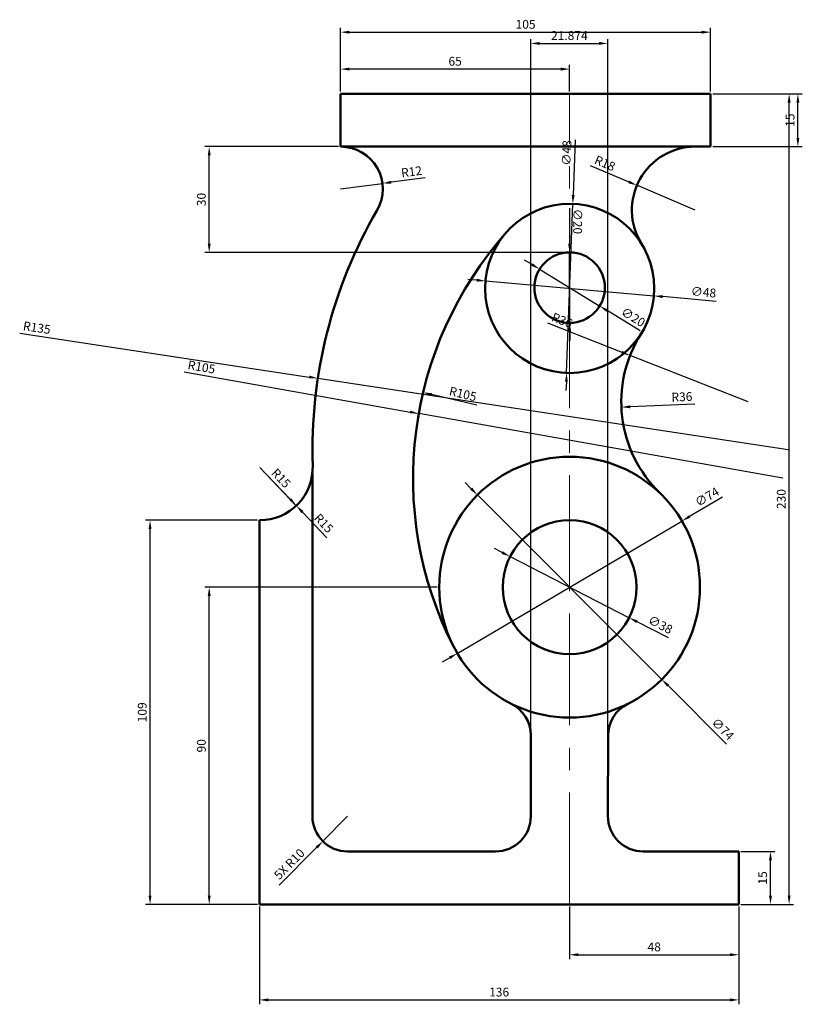
# Model space of a CAD drawing. Units: millimetres. Extents: x 3631 to 150643, y 1395 to 1701.
# Tile 1 of 1: x 3631.2 to 3853.3, y 1421.4 to 1700.8. Entities that reach past the tile are written whole.
import ezdxf

# ---------------------------------------------------------------- set-up
doc = ezdxf.new("R2010")
doc.units = ezdxf.units.MM
doc.linetypes.add('CENTER', pattern=[50.8, 31.75, -6.35, 6.35, -6.35])
for name, color, linetype, lineweight in [('M-CNTR', 4, 'CENTER', 18), ('M-CONS', 8, 'Continuous', 13), ('M-DIMS', 2, 'Continuous', 25), ('M-OUTL', 7, 'Continuous', 50)]:
    doc.layers.add(name, color=color, linetype=linetype, lineweight=lineweight)
doc.styles.get("Standard").update_dxf_attribs({"font": 'arial.ttf'})
doc.dimstyles.new('ISO-25', dxfattribs={"dimtxt": 2.5, "dimasz": 2.5, "dimexe": 1.25, "dimexo": 0.625, "dimtad": 1, "dimtxsty": 'Standard', "dimcen": 2.5, "dimadec": 0, "dimazin": 0, "dimtfac": 1, "dimtmove": 0, "dimatfit": 3, "dimfxl": 1, "dimarcsym": 0})

# ---------------------------------------------------------------- blocks, each defined once
blk = doc.blocks.new('*D1')
at = {"layer": 'Defpoints', "color": 0, "transparency": 16777216}
for p in [(3819.18, 1558.53), (3755.41, 1520.98)]:
    blk.add_point(p, dxfattribs=at)
at = {"layer": 'M-DIMS', "color": 0, "lineweight": -2, "transparency": 16777216}
for p, q in [((3830.7, 1565.31), (3821.33, 1559.79)), ((3755.41, 1520.98), (3819.18, 1558.53)), ((3753.26, 1519.71), (3751.1, 1518.44))]:
    blk.add_line(p, q, dxfattribs=at)
at = {"layer": 'M-DIMS', "color": 0, "transparency": 16777216}
for points in [[(3821.12, 1560.15), (3821.54, 1559.44), (3819.18, 1558.53)], [(3753.04, 1520.07), (3753.47, 1519.35), (3755.41, 1520.98)]]:
    blk.add_solid(points, dxfattribs=at)
at = {"layer": 'M-DIMS', "color": 0, "transparency": 16777216, "insert": (3826.45, 1565.1), "char_height": 2.5, "attachment_point": 5, "rotation": 30.49}
blk.add_mtext('∅74', dxfattribs=at)
blk = doc.blocks.new('*D2')
at = {"layer": 'Defpoints', "color": 0, "transparency": 16777216}
for p in [(3770.39, 1548.43), (3804.2, 1531.08)]:
    blk.add_point(p, dxfattribs=at)
at = {"layer": 'M-DIMS', "color": 0, "lineweight": -2, "transparency": 16777216}
for p, q in [((3768.16, 1549.57), (3765.94, 1550.71)), ((3770.39, 1548.43), (3804.2, 1531.08)), ((3815.37, 1525.35), (3806.42, 1529.94))]:
    blk.add_line(p, q, dxfattribs=at)
at = {"layer": 'M-DIMS', "color": 0, "transparency": 16777216}
for points in [[(3768.35, 1549.94), (3767.97, 1549.2), (3770.39, 1548.43)], [(3806.61, 1530.31), (3806.23, 1529.57), (3804.2, 1531.08)]]:
    blk.add_solid(points, dxfattribs=at)
at = {"layer": 'M-DIMS', "color": 0, "transparency": 16777216, "insert": (3812.91, 1528.83), "char_height": 2.5, "attachment_point": 5, "rotation": 332.8421}
blk.add_mtext('∅38', dxfattribs=at)
blk = doc.blocks.new('*D3')
at = {"layer": 'Defpoints', "color": 0, "transparency": 16777216}
for p in [(3778.77, 1629.98), (3795.82, 1619.53)]:
    blk.add_point(p, dxfattribs=at)
at = {"layer": 'M-DIMS', "color": 0, "lineweight": -2, "transparency": 16777216}
for p, q in [((3776.64, 1631.29), (3774.51, 1632.59)), ((3778.77, 1629.98), (3795.82, 1619.53)), ((3807.34, 1612.46), (3797.95, 1618.22))]:
    blk.add_line(p, q, dxfattribs=at)
at = {"layer": 'M-DIMS', "color": 0, "transparency": 16777216}
for points in [[(3776.85, 1631.64), (3776.42, 1630.93), (3778.77, 1629.98)], [(3798.17, 1618.57), (3797.73, 1617.86), (3795.82, 1619.53)]]:
    blk.add_solid(points, dxfattribs=at)
at = {"layer": 'M-DIMS', "color": 0, "transparency": 16777216, "insert": (3805.16, 1616.11), "char_height": 2.5, "attachment_point": 5, "rotation": 328.483}
blk.add_mtext('∅20', dxfattribs=at)
blk = doc.blocks.new('*D4')
at = {"layer": 'Defpoints', "color": 0, "transparency": 16777216}
for p in [(3763.42, 1626.64), (3811.23, 1622.41)]:
    blk.add_point(p, dxfattribs=at)
at = {"layer": 'M-DIMS', "color": 0, "lineweight": -2, "transparency": 16777216}
for p, q in [((3760.93, 1626.86), (3758.44, 1627.08)), ((3763.42, 1626.64), (3811.23, 1622.41)), ((3828.86, 1620.85), (3813.72, 1622.19))]:
    blk.add_line(p, q, dxfattribs=at)
at = {"layer": 'M-DIMS', "color": 0, "transparency": 16777216}
for points in [[(3760.96, 1627.28), (3760.89, 1626.45), (3763.42, 1626.64)], [(3813.76, 1622.6), (3813.68, 1621.77), (3811.23, 1622.41)]]:
    blk.add_solid(points, dxfattribs=at)
at = {"layer": 'M-DIMS', "color": 0, "transparency": 16777216, "insert": (3825.27, 1623.15), "char_height": 2.5, "attachment_point": 5, "rotation": 354.9405}
blk.add_mtext('∅48', dxfattribs=at)
blk = doc.blocks.new('*D5')
at = {"layer": 'Defpoints', "color": 0, "transparency": 16777216}
for p in [(3827.29, 1679.75), (3852.08, 1679.75), (3827.29, 1664.75)]:
    blk.add_point(p, dxfattribs=at)
at = {"layer": 'M-DIMS', "color": 0, "lineweight": -2, "transparency": 16777216}
for p, q in [((3827.92, 1679.75), (3853.33, 1679.75)), ((3852.08, 1667.25), (3852.08, 1677.25)), ((3827.92, 1664.75), (3853.33, 1664.75))]:
    blk.add_line(p, q, dxfattribs=at)
at = {"layer": 'M-DIMS', "color": 0, "transparency": 16777216}
for points in [[(3851.67, 1677.25), (3852.5, 1677.25), (3852.08, 1679.75)], [(3851.67, 1667.25), (3852.5, 1667.25), (3852.08, 1664.75)]]:
    blk.add_solid(points, dxfattribs=at)
at = {"layer": 'M-DIMS', "color": 0, "transparency": 16777216, "insert": (3850.18, 1672.25), "char_height": 2.5, "attachment_point": 5, "rotation": 90}
blk.add_mtext('15', dxfattribs=at)
blk = doc.blocks.new('*D6')
at = {"layer": 'Defpoints', "color": 0, "transparency": 16777216}
for p in [(3699.29, 1449.75), (3835.29, 1449.75), (3835.29, 1422.64)]:
    blk.add_point(p, dxfattribs=at)
at = {"layer": 'M-DIMS', "color": 0, "lineweight": -2, "transparency": 16777216}
for p, q in [((3699.29, 1449.13), (3699.29, 1421.39)), ((3835.29, 1449.13), (3835.29, 1421.39)), ((3701.79, 1422.64), (3832.79, 1422.64))]:
    blk.add_line(p, q, dxfattribs=at)
at = {"layer": 'M-DIMS', "color": 0, "transparency": 16777216}
for points in [[(3701.79, 1423.06), (3701.79, 1422.22), (3699.29, 1422.64)], [(3832.79, 1423.06), (3832.79, 1422.22), (3835.29, 1422.64)]]:
    blk.add_solid(points, dxfattribs=at)
at = {"layer": 'M-DIMS', "color": 0, "transparency": 16777216, "insert": (3767.29, 1424.54), "char_height": 2.5, "attachment_point": 5}
blk.add_mtext('136', dxfattribs=at)
blk = doc.blocks.new('*D7')
at = {"layer": 'Defpoints', "color": 0, "transparency": 16777216}
for p in [(3668.21, 1558.75), (3699.29, 1558.75), (3699.29, 1449.75)]:
    blk.add_point(p, dxfattribs=at)
at = {"layer": 'M-DIMS', "color": 0, "lineweight": -2, "transparency": 16777216}
for p, q in [((3698.67, 1558.75), (3666.96, 1558.75)), ((3668.21, 1452.25), (3668.21, 1556.25)), ((3698.67, 1449.75), (3666.96, 1449.75))]:
    blk.add_line(p, q, dxfattribs=at)
at = {"layer": 'M-DIMS', "color": 0, "transparency": 16777216}
for points in [[(3667.79, 1556.25), (3668.62, 1556.25), (3668.21, 1558.75)], [(3667.79, 1452.25), (3668.62, 1452.25), (3668.21, 1449.75)]]:
    blk.add_solid(points, dxfattribs=at)
at = {"layer": 'M-DIMS', "color": 0, "transparency": 16777216, "insert": (3666.31, 1504.25), "char_height": 2.5, "attachment_point": 5, "rotation": 90}
blk.add_mtext('109', dxfattribs=at)
blk = doc.blocks.new('*D8')
at = {"layer": 'Defpoints', "color": 0, "transparency": 16777216}
for p in [(3699.38, 1573.75), (3709.73, 1562.9)]:
    blk.add_point(p, dxfattribs=at)
at = {"layer": 'M-DIMS', "color": 0, "lineweight": -2, "transparency": 16777216}
blk.add_line((3701.28, 1571.76), (3708, 1564.71), dxfattribs=at)
at = {"layer": 'M-DIMS', "color": 0, "transparency": 16777216}
blk.add_solid([(3708.31, 1565), (3707.7, 1564.42), (3709.73, 1562.9)], dxfattribs=at)
at = {"layer": 'M-DIMS', "color": 0, "transparency": 16777216, "insert": (3705.15, 1570.45), "char_height": 2.5, "attachment_point": 5, "rotation": 313.6597}
blk.add_mtext('R15', dxfattribs=at)
blk = doc.blocks.new('*D9')
at = {"layer": 'Defpoints', "color": 0, "transparency": 16777216}
for p in [(3801.98, 1590.83), (3837.95, 1592.32)]:
    blk.add_point(p, dxfattribs=at)
at = {"layer": 'M-DIMS', "color": 0, "lineweight": -2, "transparency": 16777216}
blk.add_line((3822.85, 1591.7), (3804.48, 1590.94), dxfattribs=at)
at = {"layer": 'M-DIMS', "color": 0, "transparency": 16777216}
blk.add_solid([(3804.46, 1591.35), (3804.49, 1590.52), (3801.98, 1590.83)], dxfattribs=at)
at = {"layer": 'M-DIMS', "color": 0, "transparency": 16777216, "insert": (3819.17, 1593.45), "char_height": 2.5, "attachment_point": 5, "rotation": 2.3665}
blk.add_mtext('R36', dxfattribs=at)
blk = doc.blocks.new('*D10')
at = {"layer": 'Defpoints', "color": 0, "transparency": 16777216}
for p in [(3745.7, 1594.99), (3847.85, 1570.69)]:
    blk.add_point(p, dxfattribs=at)
at = {"layer": 'M-DIMS', "color": 0, "lineweight": -2, "transparency": 16777216}
blk.add_line((3760.96, 1591.36), (3748.13, 1594.41), dxfattribs=at)
at = {"layer": 'M-DIMS', "color": 0, "transparency": 16777216}
blk.add_solid([(3748.23, 1594.82), (3748.03, 1594.01), (3745.7, 1594.99)], dxfattribs=at)
at = {"layer": 'M-DIMS', "color": 0, "transparency": 16777216, "insert": (3756.93, 1594.27), "char_height": 2.5, "attachment_point": 5, "rotation": 346.6197}
blk.add_mtext('R105', dxfattribs=at)
blk = doc.blocks.new('*D11')
at = {"layer": 'Defpoints', "color": 0, "transparency": 16777216}
for p in [(3827.29, 1697.24), (3722.29, 1679.75), (3827.29, 1679.75)]:
    blk.add_point(p, dxfattribs=at)
at = {"layer": 'M-DIMS', "color": 0, "lineweight": -2, "transparency": 16777216}
for p, q in [((3722.29, 1680.38), (3722.29, 1698.49)), ((3724.79, 1697.24), (3824.79, 1697.24)), ((3827.29, 1680.38), (3827.29, 1698.49))]:
    blk.add_line(p, q, dxfattribs=at)
at = {"layer": 'M-DIMS', "color": 0, "transparency": 16777216}
for points in [[(3724.79, 1697.65), (3724.79, 1696.82), (3722.29, 1697.24)], [(3824.79, 1697.65), (3824.79, 1696.82), (3827.29, 1697.24)]]:
    blk.add_solid(points, dxfattribs=at)
at = {"layer": 'M-DIMS', "color": 0, "transparency": 16777216, "insert": (3774.79, 1699.14), "char_height": 2.5, "attachment_point": 5}
blk.add_mtext('105', dxfattribs=at)
blk = doc.blocks.new('*D12')
at = {"layer": 'Defpoints', "color": 0, "transparency": 16777216}
for p in [(3722.29, 1686.76), (3722.29, 1679.75), (3787.29, 1679.75)]:
    blk.add_point(p, dxfattribs=at)
at = {"layer": 'M-DIMS', "color": 0, "lineweight": -2, "transparency": 16777216}
for p, q in [((3722.29, 1680.38), (3722.29, 1688.01)), ((3787.29, 1680.38), (3787.29, 1688.01)), ((3784.79, 1686.76), (3724.79, 1686.76))]:
    blk.add_line(p, q, dxfattribs=at)
at = {"layer": 'M-DIMS', "color": 0, "transparency": 16777216}
for points in [[(3724.79, 1687.18), (3724.79, 1686.34), (3722.29, 1686.76)], [(3784.79, 1687.18), (3784.79, 1686.34), (3787.29, 1686.76)]]:
    blk.add_solid(points, dxfattribs=at)
at = {"layer": 'M-DIMS', "color": 0, "transparency": 16777216, "insert": (3754.79, 1688.66), "char_height": 2.5, "attachment_point": 5}
blk.add_mtext('65', dxfattribs=at)
blk = doc.blocks.new('*D13')
at = {"layer": 'Defpoints', "color": 0, "transparency": 16777216}
for p in [(3835.29, 1464.75), (3844.3, 1464.75), (3835.29, 1449.75)]:
    blk.add_point(p, dxfattribs=at)
at = {"layer": 'M-DIMS', "color": 0, "lineweight": -2, "transparency": 16777216}
for p, q in [((3835.92, 1464.75), (3845.55, 1464.75)), ((3844.3, 1452.25), (3844.3, 1462.25)), ((3835.92, 1449.75), (3845.55, 1449.75))]:
    blk.add_line(p, q, dxfattribs=at)
at = {"layer": 'M-DIMS', "color": 0, "transparency": 16777216}
for points in [[(3843.88, 1462.25), (3844.72, 1462.25), (3844.3, 1464.75)], [(3843.88, 1452.25), (3844.72, 1452.25), (3844.3, 1449.75)]]:
    blk.add_solid(points, dxfattribs=at)
at = {"layer": 'M-DIMS', "color": 0, "transparency": 16777216, "insert": (3842.4, 1457.25), "char_height": 2.5, "attachment_point": 5, "rotation": 90}
blk.add_mtext('15', dxfattribs=at)
blk = doc.blocks.new('*D14')
at = {"layer": 'Defpoints', "color": 0, "transparency": 16777216}
for p in [(3827.29, 1679.75), (3849.59, 1679.75), (3835.29, 1449.75)]:
    blk.add_point(p, dxfattribs=at)
at = {"layer": 'M-DIMS', "color": 0, "lineweight": -2, "transparency": 16777216}
for p, q in [((3827.92, 1679.75), (3850.84, 1679.75)), ((3849.59, 1452.25), (3849.59, 1677.25)), ((3835.92, 1449.75), (3850.84, 1449.75))]:
    blk.add_line(p, q, dxfattribs=at)
at = {"layer": 'M-DIMS', "color": 0, "transparency": 16777216}
for points in [[(3849.18, 1677.25), (3850.01, 1677.25), (3849.59, 1679.75)], [(3849.18, 1452.25), (3850.01, 1452.25), (3849.59, 1449.75)]]:
    blk.add_solid(points, dxfattribs=at)
at = {"layer": 'M-DIMS', "color": 0, "transparency": 16777216, "insert": (3847.69, 1564.75), "char_height": 2.5, "attachment_point": 5, "rotation": 90}
blk.add_mtext('230', dxfattribs=at)
blk = doc.blocks.new('*D15')
at = {"layer": 'Defpoints', "color": 0, "transparency": 16777216}
for p in [(3684.99, 1539.75), (3750.29, 1539.75), (3699.29, 1449.75)]:
    blk.add_point(p, dxfattribs=at)
at = {"layer": 'M-DIMS', "color": 0, "lineweight": -2, "transparency": 16777216}
for p, q in [((3749.67, 1539.75), (3683.74, 1539.75)), ((3684.99, 1452.25), (3684.99, 1537.25)), ((3698.67, 1449.75), (3683.74, 1449.75))]:
    blk.add_line(p, q, dxfattribs=at)
at = {"layer": 'M-DIMS', "color": 0, "transparency": 16777216}
for points in [[(3684.58, 1537.25), (3685.41, 1537.25), (3684.99, 1539.75)], [(3684.58, 1452.25), (3685.41, 1452.25), (3684.99, 1449.75)]]:
    blk.add_solid(points, dxfattribs=at)
at = {"layer": 'M-DIMS', "color": 0, "transparency": 16777216, "insert": (3683.09, 1494.75), "char_height": 2.5, "attachment_point": 5, "rotation": 90}
blk.add_mtext('90', dxfattribs=at)
blk = doc.blocks.new('*D16')
at = {"layer": 'Defpoints', "color": 0, "transparency": 16777216}
for p in [(3684.99, 1664.75), (3722.29, 1664.75), (3787.29, 1634.75)]:
    blk.add_point(p, dxfattribs=at)
at = {"layer": 'M-DIMS', "color": 0, "lineweight": -2, "transparency": 16777216}
for p, q in [((3721.67, 1664.75), (3683.74, 1664.75)), ((3684.99, 1637.25), (3684.99, 1662.25)), ((3786.67, 1634.75), (3683.74, 1634.75))]:
    blk.add_line(p, q, dxfattribs=at)
at = {"layer": 'M-DIMS', "color": 0, "transparency": 16777216}
for points in [[(3684.58, 1662.25), (3685.41, 1662.25), (3684.99, 1664.75)], [(3684.58, 1637.25), (3685.41, 1637.25), (3684.99, 1634.75)]]:
    blk.add_solid(points, dxfattribs=at)
at = {"layer": 'M-DIMS', "color": 0, "transparency": 16777216, "insert": (3683.09, 1649.75), "char_height": 2.5, "attachment_point": 5, "rotation": 90}
blk.add_mtext('30', dxfattribs=at)
blk = doc.blocks.new('*D17')
at = {"layer": 'Defpoints', "color": 0, "transparency": 16777216}
for p in [(3787.29, 1449.75), (3835.29, 1449.75), (3835.29, 1435.45)]:
    blk.add_point(p, dxfattribs=at)
at = {"layer": 'M-DIMS', "color": 0, "lineweight": -2, "transparency": 16777216}
for p, q in [((3787.29, 1449.13), (3787.29, 1434.2)), ((3835.29, 1449.13), (3835.29, 1434.2)), ((3789.79, 1435.45), (3832.79, 1435.45))]:
    blk.add_line(p, q, dxfattribs=at)
at = {"layer": 'M-DIMS', "color": 0, "transparency": 16777216}
for points in [[(3789.79, 1435.87), (3789.79, 1435.04), (3787.29, 1435.45)], [(3832.79, 1435.87), (3832.79, 1435.04), (3835.29, 1435.45)]]:
    blk.add_solid(points, dxfattribs=at)
at = {"layer": 'M-DIMS', "color": 0, "transparency": 16777216, "insert": (3811.29, 1437.35), "char_height": 2.5, "attachment_point": 5}
blk.add_mtext('48', dxfattribs=at)
blk = doc.blocks.new('*D18')
at = {"layer": 'Defpoints', "color": 0, "transparency": 16777216}
for p in [(3798.15, 1694.05), (3776.28, 1474.77), (3798.15, 1474.78)]:
    blk.add_point(p, dxfattribs=at)
at = {"layer": 'M-DIMS', "color": 0, "lineweight": -2, "transparency": 16777216}
for p, q in [((3776.28, 1475.39), (3776.28, 1695.3)), ((3778.78, 1694.05), (3795.65, 1694.05)), ((3798.15, 1475.41), (3798.15, 1695.3))]:
    blk.add_line(p, q, dxfattribs=at)
at = {"layer": 'M-DIMS', "color": 0, "transparency": 16777216}
for points in [[(3778.78, 1694.47), (3778.78, 1693.64), (3776.28, 1694.05)], [(3795.65, 1694.47), (3795.65, 1693.64), (3798.15, 1694.05)]]:
    blk.add_solid(points, dxfattribs=at)
at = {"layer": 'M-DIMS', "color": 0, "transparency": 16777216, "insert": (3787.22, 1695.95), "char_height": 2.5, "attachment_point": 5}
blk.add_mtext('21.874', dxfattribs=at)
blk = doc.blocks.new('*D19')
at = {"layer": 'Defpoints', "color": 0, "transparency": 16777216}
for p in [(3734.19, 1654.33), (3722.29, 1652.75)]:
    blk.add_point(p, dxfattribs=at)
at = {"layer": 'M-DIMS', "color": 0, "lineweight": -2, "transparency": 16777216}
for p, q in [((3722.29, 1652.75), (3734.19, 1654.33)), ((3746.28, 1655.94), (3736.67, 1654.66))]:
    blk.add_line(p, q, dxfattribs=at)
at = {"layer": 'M-DIMS', "color": 0, "transparency": 16777216}
blk.add_solid([(3736.61, 1655.07), (3736.72, 1654.25), (3734.19, 1654.33)], dxfattribs=at)
at = {"layer": 'M-DIMS', "color": 0, "transparency": 16777216, "insert": (3742.47, 1657.33), "char_height": 2.5, "attachment_point": 5, "rotation": 7.5589}
blk.add_mtext('R12', dxfattribs=at)
blk = doc.blocks.new('*D20')
at = {"layer": 'Defpoints', "color": 0, "transparency": 16777216}
for p in [(3806.39, 1653.78), (3822.96, 1646.75)]:
    blk.add_point(p, dxfattribs=at)
at = {"layer": 'M-DIMS', "color": 0, "lineweight": -2, "transparency": 16777216}
for p, q in [((3793.12, 1659.4), (3804.09, 1654.75)), ((3822.96, 1646.75), (3806.39, 1653.78))]:
    blk.add_line(p, q, dxfattribs=at)
at = {"layer": 'M-DIMS', "color": 0, "transparency": 16777216}
blk.add_solid([(3804.25, 1655.14), (3803.92, 1654.37), (3806.39, 1653.78)], dxfattribs=at)
at = {"layer": 'M-DIMS', "color": 0, "transparency": 16777216, "insert": (3797.19, 1659.74), "char_height": 2.5, "attachment_point": 5, "rotation": 337.0279}
blk.add_mtext('R18', dxfattribs=at)
blk = doc.blocks.new('*D21')
at = {"layer": 'Defpoints', "color": 0, "transparency": 16777216}
for p in [(3715.83, 1599.01), (3849.29, 1578.73)]:
    blk.add_point(p, dxfattribs=at)
at = {"layer": 'M-DIMS', "color": 0, "lineweight": -2, "transparency": 16777216}
for p, q in [((3631.2, 1611.87), (3713.35, 1599.39)), ((3849.29, 1578.73), (3715.83, 1599.01))]:
    blk.add_line(p, q, dxfattribs=at)
at = {"layer": 'M-DIMS', "color": 0, "transparency": 16777216}
blk.add_solid([(3713.42, 1599.8), (3713.29, 1598.98), (3715.83, 1599.01)], dxfattribs=at)
at = {"layer": 'M-DIMS', "color": 0, "transparency": 16777216, "insert": (3636.03, 1613.06), "char_height": 2.5, "attachment_point": 5, "rotation": 351.358}
blk.add_mtext('R135', dxfattribs=at)
blk = doc.blocks.new('*D22')
at = {"layer": 'Defpoints', "color": 0, "transparency": 16777216}
for p in [(3724.29, 1474.75), (3717.25, 1467.65)]:
    blk.add_point(p, dxfattribs=at)
at = {"layer": 'M-DIMS', "color": 0, "lineweight": -2, "transparency": 16777216}
for p, q in [((3724.29, 1474.75), (3717.25, 1467.65)), ((3704.87, 1455.16), (3715.49, 1465.88))]:
    blk.add_line(p, q, dxfattribs=at)
at = {"layer": 'M-DIMS', "color": 0, "transparency": 16777216}
blk.add_solid([(3715.2, 1466.17), (3715.79, 1465.58), (3717.25, 1467.65)], dxfattribs=at)
at = {"layer": 'M-DIMS', "color": 0, "transparency": 16777216, "insert": (3707.95, 1460.97), "char_height": 2.5, "attachment_point": 5, "rotation": 45.2458}
blk.add_mtext('5X R10', dxfattribs=at)
blk = doc.blocks.new('*D23')
at = {"layer": 'Defpoints', "color": 0, "transparency": 16777216}
for p in [(3699.38, 1573.75), (3709.71, 1562.88)]:
    blk.add_point(p, dxfattribs=at)
at = {"layer": 'M-DIMS', "color": 0, "lineweight": -2, "transparency": 16777216}
for p, q in [((3699.38, 1573.75), (3709.71, 1562.88)), ((3718.41, 1553.74), (3711.43, 1561.07))]:
    blk.add_line(p, q, dxfattribs=at)
at = {"layer": 'M-DIMS', "color": 0, "transparency": 16777216}
blk.add_solid([(3711.74, 1561.36), (3711.13, 1560.78), (3709.71, 1562.88)], dxfattribs=at)
at = {"layer": 'M-DIMS', "color": 0, "transparency": 16777216, "insert": (3717.29, 1557.67), "char_height": 2.5, "attachment_point": 5, "rotation": 313.5569}
blk.add_mtext('R15', dxfattribs=at)
blk = doc.blocks.new('*D24')
at = {"layer": 'Defpoints', "color": 0, "transparency": 16777216}
for p in [(3744.46, 1589.02), (3847.85, 1570.69)]:
    blk.add_point(p, dxfattribs=at)
at = {"layer": 'M-DIMS', "color": 0, "lineweight": -2, "transparency": 16777216}
for p, q in [((3677.91, 1600.83), (3742, 1589.46)), ((3847.85, 1570.69), (3744.46, 1589.02))]:
    blk.add_line(p, q, dxfattribs=at)
at = {"layer": 'M-DIMS', "color": 0, "transparency": 16777216}
blk.add_solid([(3742.07, 1589.87), (3741.92, 1589.05), (3744.46, 1589.02)], dxfattribs=at)
at = {"layer": 'M-DIMS', "color": 0, "transparency": 16777216, "insert": (3682.76, 1601.9), "char_height": 2.5, "attachment_point": 5, "rotation": 349.945}
blk.add_mtext('R105', dxfattribs=at)
blk = doc.blocks.new('*D25')
at = {"layer": 'Defpoints', "color": 0, "transparency": 16777216}
for p in [(3804.45, 1605.5), (3837.95, 1592.32)]:
    blk.add_point(p, dxfattribs=at)
at = {"layer": 'M-DIMS', "color": 0, "lineweight": -2, "transparency": 16777216}
for p, q in [((3780.99, 1614.73), (3802.12, 1606.42)), ((3837.95, 1592.32), (3804.45, 1605.5))]:
    blk.add_line(p, q, dxfattribs=at)
at = {"layer": 'M-DIMS', "color": 0, "transparency": 16777216}
blk.add_solid([(3802.27, 1606.8), (3801.97, 1606.03), (3804.45, 1605.5)], dxfattribs=at)
at = {"layer": 'M-DIMS', "color": 0, "transparency": 16777216, "insert": (3785.04, 1615.18), "char_height": 2.5, "attachment_point": 5, "rotation": 338.5202}
blk.add_mtext('R36', dxfattribs=at)
blk = doc.blocks.new('*D26')
at = {"layer": 'Defpoints', "color": 0, "transparency": 16777216}
for p in [(3788.2, 1648.51), (3786.45, 1600.54)]:
    blk.add_point(p, dxfattribs=at)
at = {"layer": 'M-DIMS', "color": 0, "lineweight": -2, "transparency": 16777216}
for p, q in [((3788.86, 1666.68), (3788.29, 1651.01)), ((3786.45, 1600.54), (3788.2, 1648.51)), ((3786.36, 1598.04), (3786.26, 1595.54))]:
    blk.add_line(p, q, dxfattribs=at)
at = {"layer": 'M-DIMS', "color": 0, "transparency": 16777216}
for points in [[(3787.88, 1651.02), (3788.71, 1650.99), (3788.2, 1648.51)], [(3785.94, 1598.06), (3786.77, 1598.03), (3786.45, 1600.54)]]:
    blk.add_solid(points, dxfattribs=at)
at = {"layer": 'M-DIMS', "color": 0, "transparency": 16777216, "insert": (3786.76, 1662.97), "char_height": 2.5, "attachment_point": 5, "rotation": 87.9067}
blk.add_mtext('∅48', dxfattribs=at)
blk = doc.blocks.new('*D27')
at = {"layer": 'Defpoints', "color": 0, "transparency": 16777216}
for p in [(3787.28, 1634.75), (3787.31, 1614.75)]:
    blk.add_point(p, dxfattribs=at)
at = {"layer": 'M-DIMS', "color": 0, "lineweight": -2, "transparency": 16777216}
for p, q in [((3787.26, 1647.3), (3787.28, 1637.25)), ((3787.31, 1614.75), (3787.28, 1634.75)), ((3787.31, 1612.25), (3787.31, 1609.75))]:
    blk.add_line(p, q, dxfattribs=at)
at = {"layer": 'M-DIMS', "color": 0, "transparency": 16777216}
for points in [[(3787.69, 1637.25), (3786.86, 1637.25), (3787.28, 1634.75)], [(3787.73, 1612.25), (3786.89, 1612.25), (3787.31, 1614.75)]]:
    blk.add_solid(points, dxfattribs=at)
at = {"layer": 'M-DIMS', "color": 0, "transparency": 16777216, "insert": (3789.24, 1643.53), "char_height": 2.5, "attachment_point": 5, "rotation": 270.0737}
blk.add_mtext('∅20', dxfattribs=at)
blk = doc.blocks.new('*D28')
at = {"layer": 'Defpoints', "color": 0, "transparency": 16777216}
for p in [(3761.13, 1565.92), (3813.45, 1513.59)]:
    blk.add_point(p, dxfattribs=at)
at = {"layer": 'M-DIMS', "color": 0, "lineweight": -2, "transparency": 16777216}
for p, q in [((3759.37, 1567.69), (3757.6, 1569.45)), ((3761.13, 1565.92), (3813.45, 1513.59)), ((3831.81, 1495.22), (3815.22, 1511.82))]:
    blk.add_line(p, q, dxfattribs=at)
at = {"layer": 'M-DIMS', "color": 0, "transparency": 16777216}
for points in [[(3759.66, 1567.98), (3759.07, 1567.39), (3761.13, 1565.92)], [(3815.52, 1512.11), (3814.93, 1511.52), (3813.45, 1513.59)]]:
    blk.add_solid(points, dxfattribs=at)
at = {"layer": 'M-DIMS', "color": 0, "transparency": 16777216, "insert": (3830.54, 1499.28), "char_height": 2.5, "attachment_point": 5, "rotation": 314.9935}
blk.add_mtext('∅74', dxfattribs=at)

msp = doc.modelspace()

# ---------------------------------------------------------------- linework, layer by layer
at = {"layer": 'M-CNTR'}
for p, q in [((3787.2929, 1614.7531), (3787.2929, 1679.7531)), ((3787.2929, 1539.7531), (3787.2929, 1614.7531)), ((3787.2929, 1449.7531), (3787.2929, 1539.7531))]:
    msp.add_line(p, q, dxfattribs=at)
at = {"layer": 'M-CONS'}
msp.add_line((3787.3237, 1624.5255), (3787.2929, 1624.7531), dxfattribs=at)
at = {"layer": 'M-OUTL'}
for p, q in [((3787.2929, 1679.7531), (3722.2929, 1679.7531)), ((3722.2929, 1679.7531), (3722.2929, 1664.7531)), ((3827.2929, 1679.7531), (3787.2929, 1679.7531)), ((3827.2929, 1664.7531), (3827.2929, 1679.7531)), ((3722.2929, 1664.7531), (3827.2929, 1664.7531)), ((3822.9598, 1664.7531), (3827.2929, 1664.7531)), ((3714.2929, 1474.7531), (3714.2929, 1572.1826)), ((3699.3861, 1558.7532), (3699.2929, 1558.7531)), ((3699.2929, 1449.7531), (3699.2929, 1558.7531)), ((3776.2793, 1474.7667), (3776.2481, 1497.7415)), ((3798.2194, 1497.6979), (3798.153, 1474.7821)), ((3766.2793, 1464.7531), (3724.2929, 1464.7531)), ((3835.2929, 1464.7531), (3808.153, 1464.7531)), ((3835.2929, 1449.7531), (3835.2929, 1464.7531)), ((3699.2929, 1449.7531), (3835.2929, 1449.7531))]:
    msp.add_line(p, q, dxfattribs=at)
for centre, radius in [((3787.3237, 1624.5255), 24), ((3787.2929, 1624.7531), 10), ((3787.2929, 1539.7531), 37), ((3787.2929, 1539.7531), 19)]:
    msp.add_circle(centre, radius, dxfattribs=at)
for centre, radius, start, end in [((3722.2929, 1652.7531), 12, 329.762521, 90), ((3822.9598, 1646.7531), 18, 90, 211.953423), ((3849.2929, 1578.7261), 135, 149.762521, 181.899862), ((3847.8466, 1570.6926), 105, 138.348052, 207.064399), ((3837.9471, 1592.3188), 36, 147.535404, 226.060873), ((3699.3753, 1573.7532), 15, 270.041369, 1.899862), ((3766.2481, 1497.7279), 10, 0.077771, 63.399877), ((3808.2194, 1497.6689), 10, 116.439048, 179.833968), ((3724.2929, 1474.7531), 10, 180, 270), ((3766.2793, 1474.7531), 10, 270, 0.077771), ((3808.153, 1474.7531), 10, 179.833968, 270)]:
    msp.add_arc(centre, radius, start, end, dxfattribs=at)

# ---------------------------------------------------------------- dimensions: what is measured, and where the dimension line sits
at = {"layer": 'M-DIMS'}
for base, p1, p2, override, picture, middle in [((3827.2929, 1697.2372), (3722.2929, 1679.7531), (3827.2929, 1679.7531), {"dimclrd": 0, "dimclre": 0, "dimclrt": 0}, '*D11', (3774.7929, 1699.1386)), ((3798.153, 1694.0531), (3776.2793, 1474.7667), (3798.153, 1474.7821), {"dimdec": 3, "dimlfac": 1, "dimrnd": 0, "dimzin": 0, "dimdsep": 46, "dimlunit": 2}, '*D18', (3787.2161, 1695.9546)), ((3722.2929, 1686.7588), (3787.2929, 1679.7531), (3722.2929, 1679.7531), {"dimclrd": 0, "dimclre": 0, "dimclrt": 0}, '*D12', (3754.7929, 1688.6602)), ((3835.2929, 1422.6402), (3699.2929, 1449.7531), (3835.2929, 1449.7531), {"dimclrd": 0, "dimclre": 0, "dimclrt": 0}, '*D6', (3767.2929, 1424.5425)), ((3835.2929, 1435.4531), (3787.2929, 1449.7531), (3835.2929, 1449.7531), {"dimdec": 0, "dimlfac": 1, "dimrnd": 0, "dimzin": 0, "dimdsep": 46, "dimlunit": 2}, '*D17', (3811.2929, 1437.3546))]:
    dim = msp.add_linear_dim(base=base, p1=p1, p2=p2, dimstyle='ISO-25', override=override, dxfattribs=at)
    dim.commit()
    dim.dimension.update_dxf_attribs({"geometry": picture, "text_midpoint": middle})
for base, p1, p2, override, picture, middle in [((3852.0835, 1679.7531), (3827.2929, 1664.7531), (3827.2929, 1679.7531), {"dimclrd": 0, "dimclre": 0, "dimclrt": 0}, '*D5', (3850.1821, 1672.2531)), ((3849.5929, 1679.7531), (3835.2929, 1449.7531), (3827.2929, 1679.7531), {"dimdec": 0, "dimlfac": 1, "dimrnd": 0, "dimzin": 0, "dimdsep": 46, "dimlunit": 2}, '*D14', (3847.6906, 1564.7531)), ((3684.9929, 1664.7531), (3787.2929, 1634.7531), (3722.2929, 1664.7531), {"dimdec": 0, "dimlfac": 1, "dimrnd": 0, "dimzin": 0, "dimdsep": 46, "dimlunit": 2}, '*D16', (3683.0906, 1649.7531)), ((3668.2072, 1558.7531), (3699.2929, 1449.7531), (3699.2929, 1558.7531), {"dimclrd": 0, "dimclre": 0, "dimclrt": 0}, '*D7', (3666.3058, 1504.2531)), ((3684.9929, 1539.7531), (3699.2929, 1449.7531), (3750.2929, 1539.7531), {"dimdec": 0, "dimlfac": 1, "dimrnd": 0, "dimzin": 0, "dimdsep": 46, "dimlunit": 2}, '*D15', (3683.0914, 1494.7531)), ((3844.299, 1464.7531), (3835.2929, 1449.7531), (3835.2929, 1464.7531), {"dimclrd": 0, "dimclre": 0, "dimclrt": 0}, '*D13', (3842.3975, 1457.2531))]:
    dim = msp.add_linear_dim(base=base, p1=p1, p2=p2, angle=90, dimstyle='ISO-25', override=override, dxfattribs=at)
    dim.commit()
    dim.dimension.update_dxf_attribs({"geometry": picture, "text_midpoint": middle})
for p1, p2, override, picture, middle in [((3786.4471, 1600.5415), (3788.2003, 1648.5095), {"dimdec": 0, "dimlfac": 1, "dimrnd": 0, "dimzin": 0, "dimdsep": 46, "dimlunit": 2}, '*D26', (3788.7263, 1662.8998)), ((3778.768, 1629.9806), (3795.8177, 1619.5256), {"dimclrd": 0, "dimclre": 0, "dimclrt": 0}, '*D3', (3804.1265, 1614.4305)), ((3763.4172, 1626.642), (3811.2302, 1622.4089), {"dimclrd": 0, "dimclre": 0, "dimclrt": 0}, '*D4', (3825.0946, 1621.1814)), ((3755.4093, 1520.9797), (3819.1764, 1558.5265), {"dimclrd": 0, "dimclre": 0, "dimclrt": 0}, '*D1', (3827.4516, 1563.3991)), ((3761.1329, 1565.9191), (3813.4528, 1513.5872), {"dimdec": 0, "dimlfac": 1, "dimrnd": 0, "dimzin": 0, "dimdsep": 46, "dimlunit": 2}, '*D28', (3829.1488, 1497.8876)), ((3770.3876, 1548.4256), (3804.1981, 1531.0807), {"dimclrd": 0, "dimclre": 0, "dimclrt": 0}, '*D2', (3812.0085, 1527.0739))]:
    dim = msp.add_diameter_dim_2p(p1=p1, p2=p2, dimstyle='ISO-25', override=override, dxfattribs=at)
    dim.commit()
    dim.dimension.update_dxf_attribs({"geometry": picture, "text_midpoint": middle, "dimtype": 163})
for center, mpoint, override, picture, middle in [((3822.9598, 1646.7531), (3806.3873, 1653.7782), {"dimdec": 0, "dimlfac": 1, "dimrnd": 0, "dimzin": 0, "dimdsep": 46, "dimlunit": 2}, '*D20', (3796.4438, 1657.9933)), ((3837.9471, 1592.3188), (3804.4474, 1605.501), {"dimdec": 0, "dimlfac": 1, "dimrnd": 0, "dimzin": 0, "dimdsep": 46, "dimlunit": 2}, '*D25', (3784.3476, 1613.4104)), ((3849.2929, 1578.7261), (3715.8256, 1599.0113), {"dimdec": 0, "dimlfac": 1, "dimrnd": 0, "dimzin": 0, "dimdsep": 46, "dimlunit": 2}, '*D21', (3635.7452, 1611.1824)), ((3847.8466, 1570.6926), (3744.4593, 1589.0249), {"dimdec": 0, "dimlfac": 1, "dimrnd": 0, "dimzin": 0, "dimdsep": 46, "dimlunit": 2}, '*D24', (3682.427, 1600.0244)), ((3847.8466, 1570.6926), (3745.6967, 1594.9909), {"dimclrd": 0, "dimclre": 0, "dimclrt": 0}, '*D10', (3756.4925, 1592.4229)), ((3837.9471, 1592.3188), (3801.9778, 1590.8323), {"dimclrd": 0, "dimclre": 0, "dimclrt": 0}, '*D9', (3819.247, 1591.546)), ((3699.3753, 1573.7532), (3709.7309, 1562.9014), {"dimclrd": 0, "dimclre": 0, "dimclrt": 0}, '*D8', (3703.779, 1569.1385)), ((3699.3753, 1573.7532), (3709.7114, 1562.8828), {"dimdec": 0, "dimlfac": 1, "dimrnd": 0, "dimzin": 0, "dimdsep": 46, "dimlunit": 2}, '*D23', (3715.9131, 1556.3606))]:
    dim = msp.add_radius_dim(center=center, mpoint=mpoint, dimstyle='ISO-25', override=override, dxfattribs=at)
    dim.commit()
    dim.dimension.update_dxf_attribs({"geometry": picture, "text_midpoint": middle, "dimtype": 164})
dim = msp.add_radius_dim(center=(3722.2929, 1652.7531), mpoint=(3734.1886, 1654.3317), dimstyle='ISO-25', override={"dimdec": 0, "dimlfac": 1, "dimrnd": 0, "dimzin": 0, "dimdsep": 46, "dimlunit": 2}, dxfattribs=at)
dim.commit()
dim.dimension.update_dxf_attribs({"geometry": '*D19', "text_midpoint": (3742.4656, 1657.3266)})
dim = msp.add_diameter_dim_2p(p1=(3787.3057, 1614.7531), p2=(3787.28, 1634.7531), dimstyle='ISO-25', override={"dimdec": 0, "dimlfac": 1, "dimrnd": 0, "dimzin": 0, "dimdsep": 46, "dimlunit": 2}, dxfattribs=at)
dim.commit()
dim.dimension.update_dxf_attribs({"geometry": '*D27', "text_midpoint": (3787.2687, 1643.5244)})
dim = msp.add_radius_dim(center=(3724.2929, 1474.7531), mpoint=(3717.2522, 1467.6518), text='5X <>', dimstyle='ISO-25', override={"dimdec": 0, "dimlfac": 1, "dimrnd": 0, "dimzin": 0, "dimdsep": 46, "dimlunit": 2}, dxfattribs=at)
dim.commit()
dim.dimension.update_dxf_attribs({"geometry": '*D22', "text_midpoint": (3707.9506, 1460.9706)})

doc.saveas('drawing.dxf')
